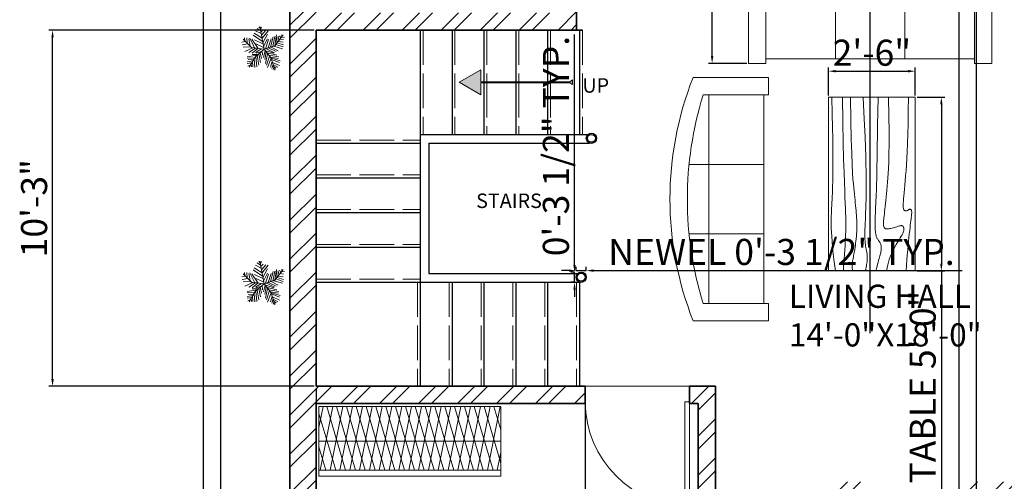
# Model space of a CAD drawing. Units: inches. Extents: x 889 to 1572, y 7262 to 8387.
# Tile 3 of 8: x 923 to 1263, y 7742 to 7901. Entities that reach past the tile are written whole.
import ezdxf

# ---------------------------------------------------------------- set-up
doc = ezdxf.new("R2010")
doc.units = ezdxf.units.IN
doc.linetypes.add('ACAD_ISO02W100', pattern=[15, 12, -3])
for name, color, linetype, lineweight in [('A-ANNO-DIMS', 2, 'Continuous', 18), ('A-ANNO-SYMB', 7, 'Continuous', 18), ('A-ANNO-TEXT', 7, 'Continuous', 18), ('A-AREA-IDEN', 7, 'Continuous', 18), ('A-DOOR', 4, 'Continuous', 18), ('A-FLOR-STRS', 7, 'Continuous', 25), ('A-FURN', 8, 'Continuous', 18), ('A-FURN-PATT', 252, 'Continuous', 13), ('A-STRS-HIDN', 8, 'ACAD_ISO02W100', 13), ('A-WALL', 7, 'Continuous', 35), ('A-WALL-PATT', 252, 'Continuous', 13), ('C-SITE', 7, 'Continuous', 30), ('L-PLNT', 94, 'Continuous', 13)]:
    doc.layers.add(name, color=color, linetype=linetype, lineweight=lineweight)
doc.styles.get("Standard").update_dxf_attribs({"font": 'arial.ttf'})
doc.dimstyles.new('ISO-25', dxfattribs={"dimtxt": 9, "dimasz": 2.5, "dimexe": 1.25, "dimexo": 0.625, "dimtad": 1, "dimlunit": 3, "dimtxsty": 'Standard', "dimcen": 2.5, "dimadec": 0, "dimazin": 0, "dimtfac": 1, "dimtmove": 0, "dimatfit": 3, "dimfxl": 1, "dimarcsym": 0})

# ---------------------------------------------------------------- blocks, each defined once
blk = doc.blocks.new('*U5')
for p, q in [((-40, 0), (-40, 6)), ((0, 0), (0, 6))]:
    blk.add_line(p, q)
blk.add_lwpolyline([(0, 0), (0, -40), (-1.75, -40), (-1.75, 0)], close=True)
blk.add_arc((0, 0), 40, 180, 270)
blk = doc.blocks.new('Sofa - Roundback 7 ft.')
for p, q in [((-12.00002, -32.4421), (-12.00003, -6.5971)), ((11.99997, -32.4421), (11.99998, -6.5971)), ((-36.000027, -34), (-36.000027, -11.4696)), ((-35.999844, -13.3819), (35.9998, -13.3819)), ((35.99998, -34), (35.99998, -11.4696)), ((-36.000027, -32.4421), (35.99998, -32.4421))]:
    blk.add_line(p, q)
for points in [[(-36.000027, -34), (-42.000027, -34), (-42.000027, -8)], [(41.99998, -8), (41.99998, -34), (35.99998, -34)]]:
    blk.add_lwpolyline(points)
for centre, radius, start, end in [((0, -114.25), 114.25, 68.43141, 111.5686), ((-0.00001, -127.1968), 121.1968, 72.72033, 107.2797)]:
    blk.add_arc(centre, radius, start, end)
blk = doc.blocks.new('Table - Rectangular Woodgrain 60 x 30 in.')
for p, q in [((0, 0), (0, -30)), ((60, 0), (0, 0)), ((60, -30), (60, 0)), ((0, -30), (60, -30))]:
    blk.add_line(p, q)
for points in [[(0, -2.4), (4.8155, -2.418), (9.0302, -2.4688), (12.709, -2.5477), (15.9167, -2.65), (18.7181, -2.7711), (21.1781, -2.9063), (23.3616, -3.0508), (25.3333, -3.2), (27.1477, -3.3495), (28.8172, -3.4958), (30.3437, -3.636), (31.7291, -3.7667), (32.9756, -3.8849), (34.0849, -3.9875), (35.059, -4.0714), (35.9, -4.1334), (36.6114, -4.1711), (37.2041, -4.1854), (37.6906, -4.1779), (38.0833, -4.15), (38.3948, -4.1034), (38.6375, -4.0396), (38.8239, -3.9602), (38.9666, -3.8667), (39.0764, -3.7608), (39.1573, -3.6448), (39.2116, -3.521), (39.2416, -3.3917), (39.2498, -3.2593), (39.2385, -3.1261), (39.21, -2.9944), (39.1666, -2.8667), (39.111, -2.7447), (39.0468, -2.6281), (38.978, -2.5163), (38.9083, -2.4083), (38.8418, -2.3035), (38.7823, -2.201), (38.7337, -2.1001), (38.7, -2), (38.6844, -1.9003), (38.6875, -1.8021), (38.7094, -1.707), (38.75, -1.6167), (38.8094, -1.5326), (38.8875, -1.4563), (38.9844, -1.3893), (39.1, -1.3333), (39.2351, -1.2896), (39.3937, -1.2583), (39.5804, -1.2396), (39.8, -1.2333), (40.057, -1.2396), (40.3562, -1.2583), (40.7023, -1.2896), (41.1, -1.3333), (41.5547, -1.3895), (42.0755, -1.4573), (42.6721, -1.5361), (43.3542, -1.625), (44.1316, -1.7233), (45.014, -1.8302), (46.0114, -1.9449), (47.1333, -2.0667), (48.3862, -2.1947), (49.7625, -2.3281), (51.2513, -2.4663), (52.8416, -2.6083), (54.5226, -2.7535), (56.2833, -2.9011), (58.1127, -3.0501), (60, -3.2)], [(0, -9.2), (6.5759, -9.0858), (11.9385, -9.0365), (16.2527, -9.0418), (19.6833, -9.0917), (22.3952, -9.1759), (24.5531, -9.2844), (26.322, -9.4069), (27.8666, -9.5333), (29.3241, -9.6553), (30.7203, -9.7719), (32.0532, -9.8837), (33.3208, -9.9917), (34.5213, -10.0965), (35.6526, -10.199), (36.7128, -10.2999), (37.7, -10.4), (38.6129, -10.4996), (39.4531, -10.5969), (40.223, -10.6895), (40.925, -10.775), (41.5613, -10.8512), (42.1344, -10.9156), (42.6465, -10.966), (43.1, -11), (43.4976, -11.0158), (43.8437, -11.0136), (44.143, -10.9942), (44.4, -10.9583), (44.6195, -10.9069), (44.8062, -10.8406), (44.9648, -10.7603), (45.1, -10.6667), (45.2155, -10.5598), (45.3114, -10.4365), (45.3871, -10.2929), (45.4416, -10.125), (45.4743, -9.929), (45.4844, -9.7011), (45.4709, -9.4371), (45.4333, -9.1333), (45.3716, -8.7883), (45.2896, -8.4104), (45.1919, -8.0107), (45.0833, -7.6), (44.9685, -7.1893), (44.8521, -6.7896), (44.7388, -6.4117), (44.6333, -6.0667), (44.54, -5.7628), (44.4614, -5.4979), (44.4001, -5.2675), (44.3583, -5.0667), (44.3384, -4.8909), (44.3427, -4.7354), (44.3736, -4.5956), (44.4333, -4.4667), (44.5236, -4.3453), (44.6427, -4.2333), (44.7884, -4.1339), (44.9583, -4.05), (45.1501, -3.9849), (45.3614, -3.9417), (45.59, -3.9234), (45.8333, -3.9333), (46.0915, -3.9749), (46.3734, -4.0531), (46.6906, -4.1736), (47.0542, -4.3417), (47.4756, -4.5629), (47.9661, -4.8427), (48.5372, -5.1866), (49.2, -5.6), (49.9676, -6.0844), (50.8594, -6.625), (51.8965, -7.2031), (53.1, -7.8), (54.491, -8.3969), (56.0906, -8.975), (57.9199, -9.5156), (60, -10)], [(0, -12.8), (5.1847, -12.9322), (9.6213, -13.0323), (13.3963, -13.1059), (16.5958, -13.1583), (19.3063, -13.1952), (21.614, -13.2219), (23.6054, -13.2439), (25.3666, -13.2667), (26.9728, -13.2947), (28.4531, -13.3281), (29.8256, -13.3663), (31.1083, -13.4083), (32.3191, -13.4535), (33.476, -13.501), (34.597, -13.5501), (35.7, -13.6), (36.7984, -13.6497), (37.8875, -13.6979), (38.9578, -13.743), (40, -13.7833), (41.0047, -13.8174), (41.9625, -13.8438), (42.864, -13.8607), (43.7, -13.8667), (44.4631, -13.8604), (45.1552, -13.8417), (45.7801, -13.8104), (46.3416, -13.7667), (46.8439, -13.7104), (47.2906, -13.6417), (47.6858, -13.5604), (48.0333, -13.4667), (48.3375, -13.3608), (48.6042, -13.2448), (48.8396, -13.121), (49.05, -12.9917), (49.2417, -12.8593), (49.4208, -12.7261), (49.5937, -12.5944), (49.7667, -12.4667), (49.9452, -12.3451), (50.1323, -12.2313), (50.3303, -12.1268), (50.5416, -12.0333), (50.7686, -11.9524), (51.0135, -11.8854), (51.2788, -11.8341), (51.5666, -11.8), (51.8785, -11.7843), (52.2116, -11.7865), (52.562, -11.8059), (52.926, -11.8417), (53.2998, -11.8931), (53.6795, -11.9594), (54.0614, -12.0397), (54.4416, -12.1333), (54.8223, -12.2401), (55.2293, -12.3625), (55.6942, -12.5037), (56.2489, -12.6667), (56.9251, -12.8547), (57.7545, -13.0708), (58.7689, -13.3182), (60, -13.6)], [(0, -18), (5.124, -17.7273), (9.6609, -17.5057), (13.6705, -17.3303), (17.2125, -17.1958), (20.3467, -17.0973), (23.1328, -17.0297), (25.6307, -16.9878), (27.9, -16.9667), (29.9928, -16.9617), (31.9302, -16.9703), (33.7254, -16.9907), (35.3917, -17.0208), (36.9423, -17.0588), (38.3906, -17.1026), (39.7499, -17.1503), (41.0333, -17.2), (42.2519, -17.2496), (43.4073, -17.2969), (44.4986, -17.3395), (45.525, -17.375), (46.4858, -17.4012), (47.3802, -17.4156), (48.2074, -17.416), (48.9667, -17.4), (49.6583, -17.3662), (50.2872, -17.3167), (50.8595, -17.2547), (51.3812, -17.1833), (51.8584, -17.1057), (52.2971, -17.025), (52.7034, -16.9443), (53.0833, -16.8667), (53.443, -16.7951), (53.789, -16.7313), (54.128, -16.6768), (54.4666, -16.6334), (54.8115, -16.6024), (55.1693, -16.5854), (55.5465, -16.5841), (55.95, -16.6), (56.3828, -16.6337), (56.8346, -16.6823), (57.2915, -16.7418), (57.7396, -16.8084), (58.165, -16.878), (58.5539, -16.9469), (58.8924, -17.0111), (59.1666, -17.0667), (59.3679, -17.1107), (59.5078, -17.1438), (59.6032, -17.1675), (59.6708, -17.1833), (59.7275, -17.193), (59.7901, -17.1979), (59.8753, -17.1998), (60, -17.2)], [(0, -22.4), (8.0098, -22.2501), (14.4094, -22.1011), (19.4168, -21.9535), (23.25, -21.8083), (26.1269, -21.6663), (28.2656, -21.5281), (29.884, -21.3947), (31.2, -21.2667), (32.3967, -21.1448), (33.5172, -21.0292), (34.5697, -20.9198), (35.5625, -20.8167), (36.5037, -20.7198), (37.4015, -20.6292), (38.2642, -20.5448), (39.1, -20.4667), (39.9164, -20.3951), (40.7187, -20.3313), (41.5117, -20.2768), (42.3, -20.2333), (43.0883, -20.2024), (43.8812, -20.1854), (44.6836, -20.1841), (45.5, -20.2), (46.3328, -20.234), (47.1747, -20.2844), (48.0163, -20.3488), (48.8479, -20.425), (49.66, -20.5106), (50.4429, -20.6031), (51.1872, -20.7004), (51.8833, -20.8), (52.5246, -20.8999), (53.1166, -20.9995), (53.6681, -21.0983), (54.1875, -21.1958), (54.6834, -21.2919), (55.1646, -21.3859), (55.6394, -21.4777), (56.1167, -21.5667), (56.6028, -21.6515), (57.0961, -21.7266), (57.5929, -21.7852), (58.0896, -21.8208), (58.5823, -21.8268), (59.0674, -21.7964), (59.5412, -21.723), (60, -21.6)], [(0, -25.2), (8.6355, -25.0504), (15.7026, -24.9031), (21.4049, -24.7606), (25.9458, -24.625), (29.529, -24.4988), (32.3578, -24.3844), (34.6359, -24.284), (36.5667, -24.2), (38.3213, -24.1341), (39.9417, -24.0854), (41.437, -24.0523), (42.8167, -24.0333), (44.0901, -24.0268), (45.2667, -24.0313), (46.3557, -24.0451), (47.3667, -24.0667), (48.309, -24.0947), (49.1928, -24.1287), (50.0284, -24.168), (50.826, -24.2125), (51.5959, -24.2617), (52.3483, -24.3151), (53.0935, -24.3725), (53.8417, -24.4334), (54.6009, -24.497), (55.3699, -24.561), (56.1454, -24.6226), (56.9239, -24.6792), (57.7021, -24.7279), (58.4764, -24.7662), (59.2435, -24.7911), (60, -24.8)], [(0, -28.8), (5.6867, -28.6681), (10.45, -28.5698), (14.407, -28.5012), (17.675, -28.4584), (20.3711, -28.4374), (22.6125, -28.4344), (24.5164, -28.4455), (26.2, -28.4667), (27.762, -28.4947), (29.2276, -28.5281), (30.6033, -28.5663), (31.8958, -28.6084), (33.1118, -28.6535), (34.2578, -28.7011), (35.3405, -28.7501), (36.3666, -28.8), (37.3443, -28.8497), (38.288, -28.8974), (39.2137, -28.9412), (40.1375, -28.9792), (41.0753, -29.0093), (42.0432, -29.0297), (43.0572, -29.0384), (44.1333, -29.0333), (45.2936, -29.0114), (46.5843, -28.9641), (48.0579, -28.8816), (49.7666, -28.7542), (51.7629, -28.5721), (54.0989, -28.3255), (56.8272, -28.0048), (60, -27.6)]]:
    blk.add_lwpolyline(points)
blk = doc.blocks.new('*U15')
for p, q in [((-8.737, 47.138), (-17.069, 52.711)), ((-10.186, 53.64), (-13.084, 55.962)), ((0, 0), (-10.5, 57)), ((-9.099, 51.782), (-6.563, 55.962)), ((-31.5, 4.5), (-52.5, 25.5)), ((-48.585, 21.131), (-49.309, 29.026)), ((-43.513, 28.561), (-42.427, 15.558)), ((-38.442, 26.239), (-34.819, 7.663)), ((-35.544, 28.097), (-24.314, 3.947)), ((-14.533, 2.09), (-30.834, 25.31)), ((-3.665, 19.273), (-27.574, 35.527)), ((-5.114, 28.097), (-24.676, 40.636)), ((-7.288, 39.707), (-21.778, 46.673)), ((-7.65, 43.423), (-2.578, 49.46)), ((-5.839, 35.992), (4.667, 48.067)), ((-5.114, 27.632), (10.463, 46.673)), ((-2.941, 16.486), (8.652, 37.85)), ((-1.129, 6.734), (9.014, 26.704)), ((10.101, 3.483), (17.708, 26.239)), ((16.259, 5.805), (23.142, 31.348)), ((22.055, 7.198), (27.489, 32.277)), ((27, 9), (48, 36)), ((27.127, 9.056), (31.112, 35.992)), ((31.836, 30.883), (32.561, 16.486)), ((35.096, 32.741), (37.27, 22.524)), ((38.719, 34.134), (41.979, 28.561)), ((40.53, 25.775), (48.862, 24.846)), ((43.791, 29.954), (51.036, 30.883)), ((44.153, 36.456), (45.239, 32.741)), ((-47.498, 19.737), (-55.83, 18.344)), ((-40.615, 13.7), (-55.105, 10.913)), ((-33.37, 6.269), (-52.207, 5.34)), ((-28.299, 3.483), (-47.86, -5.805)), ((-21.416, 3.018), (-38.079, -8.128)), ((0, 0), (-31.5, 4.5)), ((-15.982, 2.09), (-30.11, -9.521)), ((-24.314, 23.917), (-2.941, 13.7)), ((0, 0), (-22.5, -19.5)), ((-6.563, 1.161), (-21.416, -8.128)), ((-20.691, 13.7), (-1.129, 4.876)), ((0, 0), (27, 9)), ((0, 0), (18, -22.5)), ((3.942, 1.625), (11.187, 24.381)), ((6.478, 1.625), (26.04, -8.592)), ((11.187, 3.483), (30.749, -5.805)), ((18.07, 5.805), (35.096, -3.483)), ((24.229, 7.663), (46.688, 1.625)), ((29.662, 12.307), (48.137, 6.269)), ((33.285, 16.486), (48.862, 10.913)), ((36.183, 19.737), (48.137, 17.88)), ((-17.431, -15.094), (-42.789, -18.809)), ((-24.314, -21.596), (-42.427, -22.06)), ((-22.5, -19.5), (-37.5, -45)), ((-15.257, -12.772), (-30.11, -12.772)), ((-25.038, -23.918), (-22.865, -45.281)), ((-20.691, -18.345), (-17.793, -44.352)), ((-6.563, -5.805), (-19.967, -9.985)), ((-17.069, -15.094), (-12.721, -40.172)), ((-13.446, -11.378), (-8.737, -32.741)), ((-9.461, -8.592), (-6.201, -23.453)), ((-4.752, -3.483), (-3.665, -14.629)), ((2.493, -3.019), (-1.491, -20.202)), ((1.769, -2.555), (24.229, -9.521)), ((5.029, -6.27), (2.131, -25.775)), ((9.014, -11.378), (3.58, -35.992)), ((14.085, -16.951), (6.478, -40.172)), ((7.565, -9.056), (32.198, -14.629)), ((18.07, -22.524), (8.289, -45.745)), ((12.274, -15.094), (36.907, -18.809)), ((16.259, -19.738), (36.183, -22.989)), ((18, -22.5), (27, -52.5)), ((18.433, -22.524), (40.53, -29.026)), ((-28.299, -29.026), (-42.789, -31.348)), ((-30.834, -34.135), (-42.427, -35.528)), ((-34.457, -39.708), (-40.978, -42.494)), ((-26.849, -26.24), (-40.253, -25.775)), ((-32.646, -36.921), (-31.921, -44.352)), ((-29.023, -30.884), (-27.936, -43.887)), ((20.244, -30.419), (15.897, -44.816)), ((19.157, -25.311), (38.719, -33.206)), ((22.78, -37.85), (19.519, -48.532)), ((21.331, -32.741), (39.081, -40.636)), ((22.78, -38.314), (34.372, -44.816)), ((24.591, -45.745), (23.142, -50.854)), ((24.591, -43.423), (30.749, -47.603)), ((26.764, -49.925), (28.213, -50.854))]:
    blk.add_line(p, q)
blk = doc.blocks.new('STAIR-NEWEL')
for radius in [1.76, 1.36]:
    blk.add_circle((1.76, 1.76), radius)
blk = doc.blocks.new('*D60')
at = {"layer": 'A-ANNO-DIMS', "color": 0, "lineweight": -2, "transparency": 16777216}
for p, q in [((1161.87, 7922.92), (1161.87, 8002.5)), ((1173.84, 7922.92), (1160.62, 7922.92)), ((1161.87, 7888.76), (1161.87, 7920.42)), ((1173.84, 7886.26), (1160.62, 7886.26))]:
    blk.add_line(p, q, dxfattribs=at)
at = {"layer": 'A-ANNO-DIMS', "color": 0, "transparency": 16777216}
for points in [[(1161.45, 7920.42), (1162.28, 7920.42), (1161.87, 7922.92)], [(1161.45, 7888.76), (1162.28, 7888.76), (1161.87, 7886.26)]]:
    blk.add_solid(points, dxfattribs=at)
at = {"layer": 'Defpoints', "color": 0, "transparency": 16777216}
for p in [(1161.87, 7922.92), (1174.47, 7922.92), (1174.47, 7886.26)]:
    blk.add_point(p, dxfattribs=at)
at = {"layer": 'A-ANNO-DIMS', "color": 0, "transparency": 16777216, "insert": (1156.58, 7963.96), "char_height": 9, "attachment_point": 5, "rotation": 90}
blk.add_mtext('3\'-0 1/2" TYP.', dxfattribs=at)
blk = doc.blocks.new('*D63')
at = {"layer": 'A-ANNO-DIMS', "color": 0, "lineweight": -2, "transparency": 16777216}
for p, q in [((1114.88, 7814.77), (1114.88, 7815.93)), ((1118.4, 7814.77), (1118.4, 7815.93)), ((1112.38, 7814.68), (1109.88, 7814.68)), ((1114.88, 7814.68), (1118.4, 7814.68)), ((1120.9, 7814.68), (1248.25, 7814.68))]:
    blk.add_line(p, q, dxfattribs=at)
at = {"layer": 'A-ANNO-DIMS', "color": 0, "transparency": 16777216}
for points in [[(1112.38, 7815.09), (1112.38, 7814.26), (1114.88, 7814.68)], [(1120.9, 7815.09), (1120.9, 7814.26), (1118.4, 7814.68)]]:
    blk.add_solid(points, dxfattribs=at)
at = {"layer": 'Defpoints', "color": 0, "transparency": 16777216}
for p in [(1114.88, 7814.15), (1118.4, 7814.68), (1118.4, 7814.15)]:
    blk.add_point(p, dxfattribs=at)
at = {"layer": 'A-ANNO-DIMS', "color": 0, "transparency": 16777216, "insert": (1185.82, 7819.96), "char_height": 9, "attachment_point": 5}
blk.add_mtext('NEWEL 0\'-3 1/2" TYP.', dxfattribs=at)
blk = doc.blocks.new('*D64')
at = {"layer": 'A-ANNO-DIMS', "color": 0, "lineweight": -2, "transparency": 16777216}
for p, q in [((1114.35, 7816.65), (1114.35, 7896.23)), ((1114.25, 7814.15), (1113.1, 7814.15)), ((1114.35, 7810.63), (1114.35, 7814.15)), ((1114.25, 7810.63), (1113.1, 7810.63)), ((1114.35, 7808.13), (1114.35, 7805.63))]:
    blk.add_line(p, q, dxfattribs=at)
at = {"layer": 'A-ANNO-DIMS', "color": 0, "transparency": 16777216}
for points in [[(1113.93, 7816.65), (1114.77, 7816.65), (1114.35, 7814.15)], [(1113.93, 7808.13), (1114.77, 7808.13), (1114.35, 7810.63)]]:
    blk.add_solid(points, dxfattribs=at)
at = {"layer": 'Defpoints', "color": 0, "transparency": 16777216}
for p in [(1114.35, 7814.15), (1114.88, 7814.15), (1114.88, 7810.63)]:
    blk.add_point(p, dxfattribs=at)
at = {"layer": 'A-ANNO-DIMS', "color": 0, "transparency": 16777216, "insert": (1109.07, 7857.69), "char_height": 9, "attachment_point": 5, "rotation": 90}
blk.add_mtext('0\'-3 1/2" TYP.', dxfattribs=at)
blk = doc.blocks.new('*D67')
at = {"layer": 'A-ANNO-DIMS', "color": 0, "lineweight": -2, "transparency": 16777216}
for p, q in [((1232.68, 7874.55), (1242.3, 7874.55)), ((1241.05, 7872.05), (1241.05, 7817.05)), ((1232.68, 7814.55), (1242.3, 7814.55)), ((1241.05, 7814.55), (1241.05, 7689.17))]:
    blk.add_line(p, q, dxfattribs=at)
at = {"layer": 'A-ANNO-DIMS', "color": 0, "transparency": 16777216}
for points in [[(1240.64, 7872.05), (1241.47, 7872.05), (1241.05, 7874.55)], [(1240.64, 7817.05), (1241.47, 7817.05), (1241.05, 7814.55)]]:
    blk.add_solid(points, dxfattribs=at)
at = {"layer": 'Defpoints', "color": 0, "transparency": 16777216}
for p in [(1232.05, 7874.55), (1232.05, 7814.55), (1241.05, 7814.55)]:
    blk.add_point(p, dxfattribs=at)
at = {"layer": 'A-ANNO-DIMS', "color": 0, "transparency": 16777216, "insert": (1235.77, 7750.61), "char_height": 9, "attachment_point": 5, "rotation": 90}
blk.add_mtext('COFFEE TABLE 5\'-0"', dxfattribs=at)
blk = doc.blocks.new('*D68')
at = {"layer": 'A-ANNO-DIMS', "color": 0, "lineweight": -2, "transparency": 16777216}
for p, q in [((1202.05, 7875.18), (1202.05, 7884.8)), ((1232.05, 7875.18), (1232.05, 7884.8)), ((1204.55, 7883.55), (1229.55, 7883.55))]:
    blk.add_line(p, q, dxfattribs=at)
at = {"layer": 'A-ANNO-DIMS', "color": 0, "transparency": 16777216}
for points in [[(1204.55, 7883.97), (1204.55, 7883.13), (1202.05, 7883.55)], [(1229.55, 7883.97), (1229.55, 7883.13), (1232.05, 7883.55)]]:
    blk.add_solid(points, dxfattribs=at)
at = {"layer": 'Defpoints', "color": 0, "transparency": 16777216}
for p in [(1232.05, 7883.55), (1202.05, 7874.55), (1232.05, 7874.55)]:
    blk.add_point(p, dxfattribs=at)
at = {"layer": 'A-ANNO-DIMS', "color": 0, "transparency": 16777216, "insert": (1217.05, 7888.77), "char_height": 9, "attachment_point": 5}
blk.add_mtext('2\'-6"', dxfattribs=at)
blk = doc.blocks.new('*D74')
at = {"layer": 'A-ANNO-DIMS', "color": 0, "lineweight": -2, "transparency": 16777216}
for p, q in [((1247.05, 8161.11), (1247.05, 7262.35)), ((1253.05, 8161.11), (1253.05, 7262.35)), ((1244.55, 7263.6), (1242.05, 7263.6)), ((1247.05, 7263.6), (1253.05, 7263.6)), ((1255.55, 7263.6), (1283.22, 7263.6))]:
    blk.add_line(p, q, dxfattribs=at)
at = {"layer": 'A-ANNO-DIMS', "color": 0, "transparency": 16777216}
for points in [[(1244.55, 7264.02), (1244.55, 7263.19), (1247.05, 7263.6)], [(1255.55, 7264.02), (1255.55, 7263.19), (1253.05, 7263.6)]]:
    blk.add_solid(points, dxfattribs=at)
at = {"layer": 'Defpoints', "color": 0, "transparency": 16777216}
for p in [(1247.05, 8161.73), (1253.05, 8161.73), (1253.05, 7263.6)]:
    blk.add_point(p, dxfattribs=at)
at = {"layer": 'A-ANNO-DIMS', "color": 0, "transparency": 16777216, "insert": (1270.64, 7268.82), "char_height": 9, "attachment_point": 5}
blk.add_mtext('0\'-6"', dxfattribs=at)
blk = doc.blocks.new('*D75')
at = {"layer": 'A-ANNO-DIMS', "color": 0, "lineweight": -2, "transparency": 16777216}
for p, q in [((1024.42, 7897.73), (932.8, 7897.73)), ((934.05, 7777.23), (934.05, 7895.23)), ((1024.42, 7774.73), (932.8, 7774.73))]:
    blk.add_line(p, q, dxfattribs=at)
at = {"layer": 'A-ANNO-DIMS', "color": 0, "transparency": 16777216}
for points in [[(933.63, 7895.23), (934.47, 7895.23), (934.05, 7897.73)], [(933.63, 7777.23), (934.47, 7777.23), (934.05, 7774.73)]]:
    blk.add_solid(points, dxfattribs=at)
at = {"layer": 'Defpoints', "color": 0, "transparency": 16777216}
for p in [(934.05, 7897.73), (1025.05, 7897.73), (1025.05, 7774.73)]:
    blk.add_point(p, dxfattribs=at)
at = {"layer": 'A-ANNO-DIMS', "color": 0, "transparency": 16777216, "insert": (928.83, 7836.23), "char_height": 9, "attachment_point": 5, "rotation": 90}
blk.add_mtext('10\'-3"', dxfattribs=at)
blk = doc.blocks.new('*D76')
at = {"layer": 'A-ANNO-DIMS', "color": 0, "lineweight": -2, "transparency": 16777216}
for p, q in [((1025.05, 7774.11), (1025.05, 7262.35)), ((1118.05, 7774.11), (1118.05, 7262.35)), ((1027.55, 7263.6), (1115.55, 7263.6))]:
    blk.add_line(p, q, dxfattribs=at)
at = {"layer": 'A-ANNO-DIMS', "color": 0, "transparency": 16777216}
for points in [[(1027.55, 7264.02), (1027.55, 7263.19), (1025.05, 7263.6)], [(1115.55, 7264.02), (1115.55, 7263.19), (1118.05, 7263.6)]]:
    blk.add_solid(points, dxfattribs=at)
at = {"layer": 'Defpoints', "color": 0, "transparency": 16777216}
for p in [(1025.05, 7774.73), (1118.05, 7774.73), (1118.05, 7263.6)]:
    blk.add_point(p, dxfattribs=at)
at = {"layer": 'A-ANNO-DIMS', "color": 0, "transparency": 16777216, "insert": (1071.55, 7268.82), "char_height": 9, "attachment_point": 5}
blk.add_mtext('7\'-9"', dxfattribs=at)
blk = doc.blocks.new('*D77')
at = {"layer": 'A-ANNO-DIMS', "color": 0, "lineweight": -2, "transparency": 16777216}
for p, q in [((1216.46, 8017.11), (1216.46, 7916.76)), ((1216.47, 7793.06), (1216.46, 7914.26))]:
    blk.add_line(p, q, dxfattribs=at)
at = {"layer": 'A-ANNO-DIMS', "color": 0, "transparency": 16777216}
blk.add_solid([(1216.88, 7916.76), (1216.05, 7916.76), (1216.46, 7914.26)], dxfattribs=at)
at = {"layer": 'Defpoints', "color": 0, "transparency": 16777216}
for p in [(1216.46, 7914.26), (1216.47, 7793.06)]:
    blk.add_point(p, dxfattribs=at)
at = {"layer": 'A-ANNO-DIMS', "color": 0, "transparency": 16777216, "insert": (1221.69, 7986.98), "char_height": 9, "attachment_point": 5, "rotation": 270.0001}
blk.add_mtext('2X R10\'-1"', dxfattribs=at)
blk = doc.blocks.new('*D78')
at = {"layer": 'A-ANNO-DIMS', "color": 0, "lineweight": -2, "transparency": 16777216}
for p, q in [((1216.46, 8025.93), (1216.46, 7922.76)), ((1216.47, 7806.01), (1216.46, 7920.26))]:
    blk.add_line(p, q, dxfattribs=at)
at = {"layer": 'A-ANNO-DIMS', "color": 0, "transparency": 16777216}
blk.add_solid([(1216.88, 7922.76), (1216.05, 7922.76), (1216.46, 7920.26)], dxfattribs=at)
at = {"layer": 'Defpoints', "color": 0, "transparency": 16777216}
for p in [(1216.46, 7920.26), (1216.47, 7806.01)]:
    blk.add_point(p, dxfattribs=at)
at = {"layer": 'A-ANNO-DIMS', "color": 0, "transparency": 16777216, "insert": (1221.74, 7988.81), "char_height": 9, "attachment_point": 5, "rotation": 270.0001}
blk.add_mtext('2X R9\'-6 1/2"', dxfattribs=at)

msp = doc.modelspace()

# ---------------------------------------------------------------- hatches: boundary and pattern name
at = {"layer": 'A-ANNO-SYMB'}
h = msp.add_hatch(color=256, dxfattribs=at)
h.dxf.hatch_style = 1
h.paths.add_polyline_path([(1081.979, 7879.531), (1112.766, 7879.531), (1113.691, 7878.957), (1113.691, 7880.569), (1112.718, 7879.931), (1081.979, 7879.931), (1081.979, 7884.066), (1074.471, 7879.731), (1081.979, 7875.396)])
at = {"layer": 'A-FURN-PATT'}
h = msp.add_hatch(dxfattribs=at)
h.set_pattern_fill('ANSI31', color=256, scale=1.0262954, angle=61.427996, style=0)
h.paths.add_polyline_path([(1026.049, 7745.731), (1088.869, 7745.731), (1088.869, 7767.731), (1026.049, 7767.731)])
h = msp.add_hatch(dxfattribs=at)
h.set_pattern_fill('ANSI31', color=256, scale=1.049449, angle=33.75888, style=0)
h.paths.add_polyline_path([(1026.049, 7745.731), (1088.869, 7745.731), (1088.869, 7767.731), (1026.049, 7767.731)])
at = {"layer": 'A-WALL-PATT'}
h = msp.add_hatch(dxfattribs=at)
h.set_pattern_fill('ANSI32', color=256)
h.paths.add_polyline_path([(1166.049, 7624.731), (1163.049, 7624.731), (1163.049, 7774.731), (1154.049, 7774.731), (1154.049, 7768.731), (1157.049, 7768.731), (1157.049, 7624.731), (1106.049, 7624.731), (1106.049, 7615.731), (1166.049, 7615.731), (1166.049, 7618.431)])
h.paths.add_polyline_path([(1025.049, 7666.731), (1016.049, 7666.731), (1016.049, 7615.731), (1076.049, 7615.731), (1076.049, 7624.731), (1025.049, 7624.731)])
h.paths.add_polyline_path([(1025.049, 7768.731), (1118.049, 7768.731), (1118.049, 7774.731), (1025.049, 7774.731), (1025.049, 7897.731), (1115.049, 7897.731), (1115.049, 7906.731), (1109.049, 7906.731), (1109.049, 7903.731), (1025.049, 7903.731), (1025.049, 7923.231), (1016.049, 7923.231), (1016.049, 7726.731), (1025.049, 7726.731)])
h.paths.add_polyline_path([(1436.049, 7897.731), (1427.049, 7897.731), (1427.049, 7883.374), (1436.049, 7883.374)])
h.paths.add_polyline_path([(1436.049, 7853.374), (1427.049, 7853.374), (1427.049, 7843.731), (1415.049, 7843.731), (1415.049, 7837.731), (1427.049, 7837.731), (1427.049, 7831.731), (1436.049, 7831.731)])
h.paths.add_polyline_path([(1436.049, 8010.183), (1427.049, 8010.183), (1427.049, 7970.456), (1370.049, 7970.456), (1370.049, 7963.731), (1427.049, 7963.731), (1427.049, 7957.731), (1436.049, 7957.731)])
h.paths.add_polyline_path([(1436.049, 7747.731), (1427.049, 7747.731), (1427.049, 7741.731), (1344.721, 7741.731), (1344.721, 7735.731), (1349.049, 7735.731), (1349.049, 7672.731), (1355.049, 7672.731), (1355.049, 7735.731), (1427.049, 7735.731), (1427.049, 7721.931), (1436.049, 7721.931)])
h.paths.add_polyline_path([(1436.049, 7700.931), (1427.049, 7700.931), (1427.049, 7591.731), (1355.049, 7591.731), (1355.049, 7642.731), (1349.049, 7642.731), (1349.049, 7591.731), (1310.049, 7591.731), (1310.049, 7582.731), (1436.049, 7582.731)])
h.paths.add_polyline_path([(1392.42, 8272.731), (1331.049, 8272.731), (1331.049, 8263.731), (1349.049, 8263.731), (1349.049, 8224.731), (1355.049, 8224.731), (1355.049, 8263.731), (1392.42, 8263.731)])
h.paths.add_polyline_path([(1271.049, 8272.731), (1196.736, 8272.731), (1196.736, 8263.731), (1247.049, 8263.731), (1247.049, 8203.731), (1244.049, 8203.731), (1244.049, 8197.731), (1247.049, 8197.731), (1247.049, 8161.731), (1253.049, 8161.731), (1253.049, 8185.731), (1295.049, 8185.731), (1295.049, 8191.731), (1253.049, 8191.731), (1253.049, 8263.731), (1271.049, 8263.731)])
h.paths.add_polyline_path([(1175.736, 8272.731), (1102.037, 8272.731), (1102.037, 8263.731), (1157.049, 8263.731), (1157.049, 8158.731), (1163.049, 8158.731), (1163.049, 8197.731), (1214.049, 8197.731), (1214.049, 8203.731), (1163.049, 8203.731), (1163.049, 8263.731), (1175.736, 8263.731)])
h.paths.add_polyline_path([(1072.037, 8272.731), (1016.049, 8272.731), (1016.049, 8221.731), (1025.049, 8221.731), (1025.049, 8263.731), (1072.037, 8263.731)])
h.paths.add_polyline_path([(1163.049, 8122.731), (1157.049, 8122.731), (1157.049, 8119.731), (1025.049, 8119.731), (1025.049, 8161.731), (1016.049, 8161.731), (1016.049, 8071.731), (1025.049, 8071.731), (1025.049, 8113.731), (1157.049, 8113.731), (1157.049, 8110.731), (1163.049, 8110.731)])
h.paths.add_polyline_path([(1025.049, 8011.731), (1016.049, 8011.731), (1016.049, 7944.231), (1025.049, 7944.231), (1025.049, 7963.731), (1109.049, 7963.731), (1109.049, 7936.731), (1115.049, 7936.731), (1115.049, 7963.731), (1163.049, 7963.731), (1163.049, 8074.731), (1157.049, 8074.731), (1157.049, 7969.731), (1025.049, 7969.731)])
h.paths.add_polyline_path([(1314.721, 7741.731), (1307.049, 7741.731), (1307.049, 7837.731), (1319.049, 7837.731), (1319.049, 7843.731), (1307.049, 7843.731), (1307.049, 7963.731), (1310.049, 7963.731), (1310.049, 7970.456), (1301.049, 7970.456), (1301.049, 7837.731), (1301.049, 7741.731), (1250.049, 7741.731), (1250.049, 7735.731), (1314.721, 7735.731)])
h.paths.add_polyline_path([(1211.049, 7735.731), (1214.049, 7735.731), (1214.049, 7741.731), (1205.049, 7741.731), (1205.049, 7624.731), (1202.049, 7624.731), (1202.049, 7615.731), (1205.049, 7615.731), (1205.049, 7582.731), (1250.049, 7582.731), (1250.049, 7591.731), (1211.049, 7591.731)])
h.paths.add_polyline_path([(1436.049, 8260.718), (1427.049, 8260.718), (1427.049, 8191.731), (1355.049, 8191.731), (1355.049, 8194.731), (1349.049, 8194.731), (1349.049, 8191.731), (1343.049, 8191.731), (1343.049, 8185.731), (1427.049, 8185.731), (1427.049, 8070.183), (1436.049, 8070.183)])

# ---------------------------------------------------------------- linework, layer by layer
at = {"layer": 'A-ANNO-SYMB'}
for p, q in [((1113.691, 7880.569), (1112.718, 7879.931)), ((1113.691, 7880.569), (1113.691, 7878.957)), ((1112.718, 7879.931), (1081.979, 7879.931)), ((1112.766, 7879.531), (1081.979, 7879.531)), ((1113.691, 7878.957), (1112.766, 7879.531))]:
    msp.add_line(p, q, dxfattribs=at)
msp.add_lwpolyline([(1081.979, 7879.931), (1081.979, 7884.066), (1074.471, 7879.731), (1081.979, 7875.396), (1081.979, 7879.531)], dxfattribs=at)
at = {"layer": 'A-DOOR'}
msp.add_line((1154.049, 7774.731), (1118.049, 7774.731), dxfattribs=at)
at = {"layer": 'A-FLOR-STRS'}
for p, q in [((1061.049, 7897.731), (1061.049, 7774.731)), ((1072.049, 7897.731), (1072.049, 7861.731)), ((1083.049, 7897.731), (1083.049, 7879.931)), ((1094.049, 7897.731), (1094.049, 7879.931)), ((1105.049, 7897.731), (1105.049, 7879.931)), ((1116.049, 7897.731), (1116.049, 7861.731)), ((1083.049, 7879.531), (1083.049, 7861.731)), ((1094.049, 7879.531), (1094.049, 7861.731)), ((1105.049, 7879.531), (1105.049, 7861.731)), ((1061.049, 7861.731), (1119.061, 7861.731)), ((1025.049, 7858.731), (1061.049, 7858.731)), ((1064.049, 7858.731), (1119.548, 7858.731)), ((1064.049, 7858.731), (1064.049, 7813.731)), ((1025.049, 7846.731), (1061.049, 7846.731)), ((1025.049, 7834.731), (1061.049, 7834.731)), ((1025.049, 7822.731), (1061.049, 7822.731)), ((1064.049, 7813.731), (1115.5, 7813.731)), ((1025.049, 7810.731), (1116.049, 7810.731)), ((1072.049, 7810.731), (1072.049, 7774.731)), ((1083.049, 7810.731), (1083.049, 7774.731)), ((1094.049, 7810.731), (1094.049, 7774.731)), ((1105.049, 7810.731), (1105.049, 7774.731)), ((1116.049, 7810.731), (1116.049, 7774.731))]:
    msp.add_line(p, q, dxfattribs=at)
at = {"layer": 'A-FURN'}
for p, q in [((1026.049, 7767.731), (1088.869, 7767.731)), ((1026.049, 7767.731), (1026.049, 7743.731)), ((1088.869, 7767.731), (1088.869, 7743.731)), ((1026.049, 7755.731), (1088.869, 7755.731)), ((1026.049, 7745.731), (1088.869, 7745.731)), ((1026.049, 7743.731), (1088.869, 7743.731))]:
    msp.add_line(p, q, dxfattribs=at)
at = {"layer": 'A-STRS-HIDN'}
for p, q in [((1062.049, 7897.731), (1062.049, 7861.731)), ((1073.049, 7897.731), (1073.049, 7861.731)), ((1084.049, 7897.731), (1084.049, 7879.931)), ((1095.049, 7897.731), (1095.049, 7879.931)), ((1106.049, 7897.731), (1106.049, 7879.931)), ((1117.049, 7897.731), (1117.049, 7861.731)), ((1084.049, 7879.531), (1084.049, 7861.731)), ((1095.049, 7879.531), (1095.049, 7861.731)), ((1106.049, 7879.531), (1106.049, 7861.731)), ((1025.049, 7859.731), (1061.049, 7859.731)), ((1025.049, 7847.731), (1061.049, 7847.731)), ((1025.049, 7835.731), (1061.049, 7835.731)), ((1025.049, 7823.731), (1061.049, 7823.731)), ((1025.049, 7811.731), (1061.049, 7811.731)), ((1060.049, 7810.731), (1060.049, 7774.731)), ((1071.049, 7810.731), (1071.049, 7774.731)), ((1082.049, 7810.731), (1082.049, 7774.731)), ((1093.049, 7810.731), (1093.049, 7774.731)), ((1104.049, 7810.731), (1104.049, 7774.731)), ((1115.049, 7810.731), (1115.049, 7774.731))]:
    msp.add_line(p, q, dxfattribs=at)
at = {"layer": 'A-WALL'}
for p, q in [((1016.049, 8272.731), (1016.049, 7393.731)), ((1115.049, 7906.731), (1115.049, 7897.731)), ((1025.049, 7897.731), (1117.049, 7897.731)), ((1025.049, 7897.731), (1025.049, 7774.731)), ((1025.049, 7774.731), (1118.049, 7774.731)), ((1118.049, 7768.731), (1118.049, 7774.731)), ((1154.049, 7768.731), (1154.049, 7774.731)), ((1154.049, 7774.731), (1163.049, 7774.731)), ((1163.049, 7774.731), (1163.049, 7624.731)), ((1025.049, 7768.731), (1118.049, 7768.731)), ((1025.049, 7768.731), (1025.049, 7624.731)), ((1154.049, 7768.731), (1157.049, 7768.731)), ((1157.049, 7768.731), (1157.049, 7624.731))]:
    msp.add_line(p, q, dxfattribs=at)
at = {"layer": 'C-SITE'}
for p, q in [((986.049, 8272.731), (986.049, 7393.731)), ((992.049, 8272.731), (992.049, 7405.731))]:
    msp.add_line(p, q, dxfattribs=at)

# ---------------------------------------------------------------- block references
at = {"layer": 'A-DOOR', "xscale": 0.9, "yscale": 0.9, "zscale": 0.9}
msp.add_blockref('*U5', (1154.049, 7769.331), dxfattribs=at)
at = {"layer": 'A-FLOR-STRS'}
for p in [(1118.421, 7858.613), (1114.879, 7810.629)]:
    msp.add_blockref('STAIR-NEWEL', p, dxfattribs=at)
at = {"layer": 'A-FURN'}
msp.add_blockref('Sofa - Roundback 7 ft.', (1216.465, 7920.258), dxfattribs=at)
for name, p, rotation in [('Sofa - Roundback 7 ft.', (1147.309, 7839.365), 90), ('Table - Rectangular Woodgrain 60 x 30 in.', (1232.053, 7874.55), 270)]:
    msp.add_blockref(name, p, dxfattribs=dict(at, rotation=rotation))
at = {"layer": 'L-PLNT', "xscale": 0.137481440781912, "yscale": 0.137481440781912, "zscale": 0.137481440781912}
for p in [(1007.095, 7891.105), (1007.095, 7810.09)]:
    msp.add_blockref('*U15', p, dxfattribs=at)

# ---------------------------------------------------------------- texts
at = {"layer": 'A-ANNO-TEXT', "insert": (1117.049, 7881.129), "char_height": 5, "attachment_point": 1}
msp.add_mtext_dynamic_manual_height_columns('UP', width=10.10045, gutter_width=12.5, heights=[0], dxfattribs=at)
at = {"layer": 'A-AREA-IDEN', "attachment_point": 1}
for s, width, insert, char_height in [('STAIRS', 26.57466, (1080.362, 7841.297), 5), ('LIVING HALL\\P14\'-0"X18\'-0"', 67.7237, (1188.395, 7809.816), 8)]:
    msp.add_mtext_dynamic_manual_height_columns(s, width=width, gutter_width=12.5, heights=[0], dxfattribs=dict(at, insert=insert, char_height=char_height))

# ---------------------------------------------------------------- dimensions: what is measured, and where the dimension line sits
at = {"layer": 'A-ANNO-DIMS'}
for base, p1, p2, picture, middle in [((1253.049, 7263.604), (1247.049, 8161.731), (1253.049, 8161.731), '*D74', (1270.636, 7268.824)), ((1232.053, 7883.55), (1202.053, 7874.55), (1232.053, 7874.55), '*D68', (1217.053, 7888.771)), ((1118.049, 7263.604), (1025.049, 7774.731), (1118.049, 7774.731), '*D76', (1071.549, 7268.824))]:
    dim = msp.add_linear_dim(base=base, p1=p1, p2=p2, dimstyle='ISO-25', override={"dimdec": 1, "dimlfac": 1, "dimrnd": 0, "dimzin": 1, "dimdsep": 46, "dimlunit": 4, "dimfrac": 2}, dxfattribs=at)
    dim.commit()
    dim.dimension.update_dxf_attribs({"geometry": picture, "text_midpoint": middle})
for center, mpoint, picture, middle in [((1216.465178, 7806.007878), (1216.465, 7920.257878), '*D78', (1216.4648932, 7988.807878)), ((1216.465, 7793.061), (1216.465, 7914.258), '*D77', (1216.465, 7986.976))]:
    dim = msp.add_radius_dim(center=center, mpoint=mpoint, text='2X <>', dimstyle='ISO-25', override={"dimdec": 1, "dimlfac": 1, "dimrnd": 0, "dimzin": 1, "dimdsep": 46, "dimlunit": 4, "dimfrac": 2}, dxfattribs=at)
    dim.commit()
    dim.dimension.update_dxf_attribs({"geometry": picture, "text_midpoint": middle, "dimtype": 164})
for base, p1, p2, angle, text, picture, middle in [((1161.865, 7922.925), (1174.465, 7886.258), (1174.465, 7922.925), 90, '<> TYP.', '*D60', (1156.584, 7963.962)), ((1114.351, 7814.15), (1114.879, 7810.629), (1114.879, 7814.15), 90, '<> TYP.', '*D64', (1109.069, 7857.69)), ((1241.053, 7814.55), (1232.053, 7874.55), (1232.053, 7814.55), 270, 'COFFEE TABLE <>', '*D67', (1235.771, 7750.611))]:
    dim = msp.add_linear_dim(base=base, p1=p1, p2=p2, angle=angle, text=text, dimstyle='ISO-25', override={"dimdec": 1, "dimlfac": 1, "dimrnd": 0, "dimzin": 1, "dimdsep": 46, "dimlunit": 4, "dimfrac": 2}, dxfattribs=at)
    dim.commit()
    dim.dimension.update_dxf_attribs({"geometry": picture, "text_midpoint": middle})
dim = msp.add_linear_dim(base=(934.049, 7897.731), p1=(1025.049, 7774.731), p2=(1025.049, 7897.731), angle=90, dimstyle='ISO-25', override={"dimdec": 1, "dimlfac": 1, "dimrnd": 0, "dimzin": 1, "dimdsep": 46, "dimlunit": 4, "dimfrac": 2}, dxfattribs=at)
dim.commit()
dim.dimension.update_dxf_attribs({"geometry": '*D75', "text_midpoint": (928.825, 7836.231)})
dim = msp.add_linear_dim(base=(1118.4, 7814.678), p1=(1114.879, 7814.15), p2=(1118.4, 7814.15), text='NEWEL <> TYP.', dimstyle='ISO-25', override={"dimdec": 1, "dimlfac": 1, "dimrnd": 0, "dimzin": 1, "dimdsep": 46, "dimlunit": 4, "dimfrac": 2}, dxfattribs=at)
dim.commit()
dim.dimension.update_dxf_attribs({"geometry": '*D63', "text_midpoint": (1185.824, 7819.959)})

doc.saveas('drawing.dxf')
